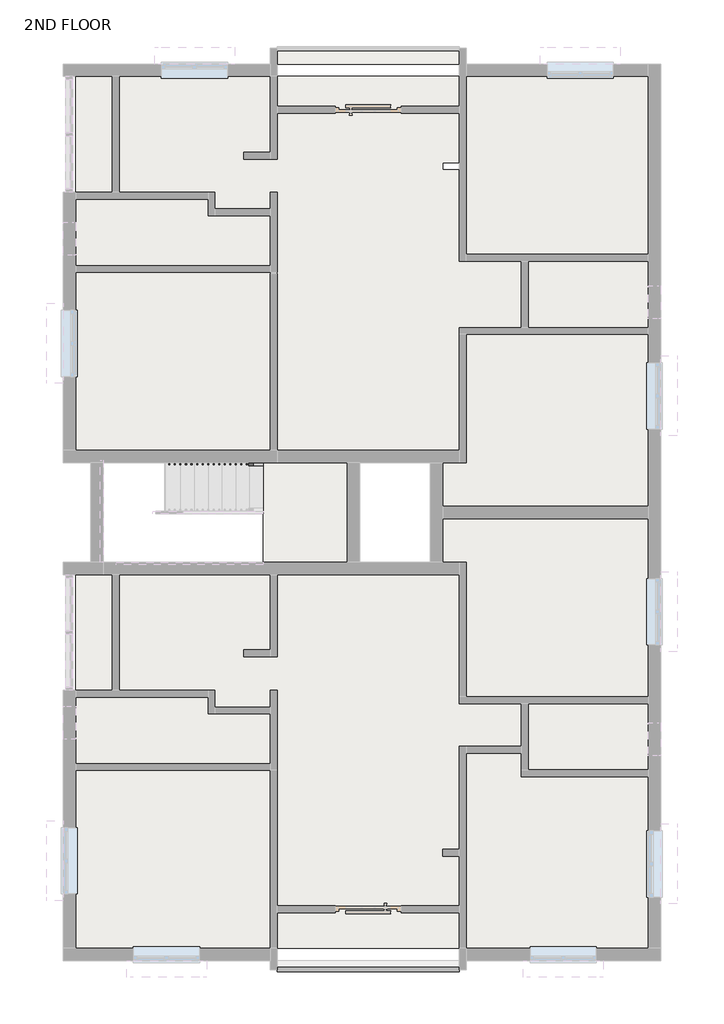
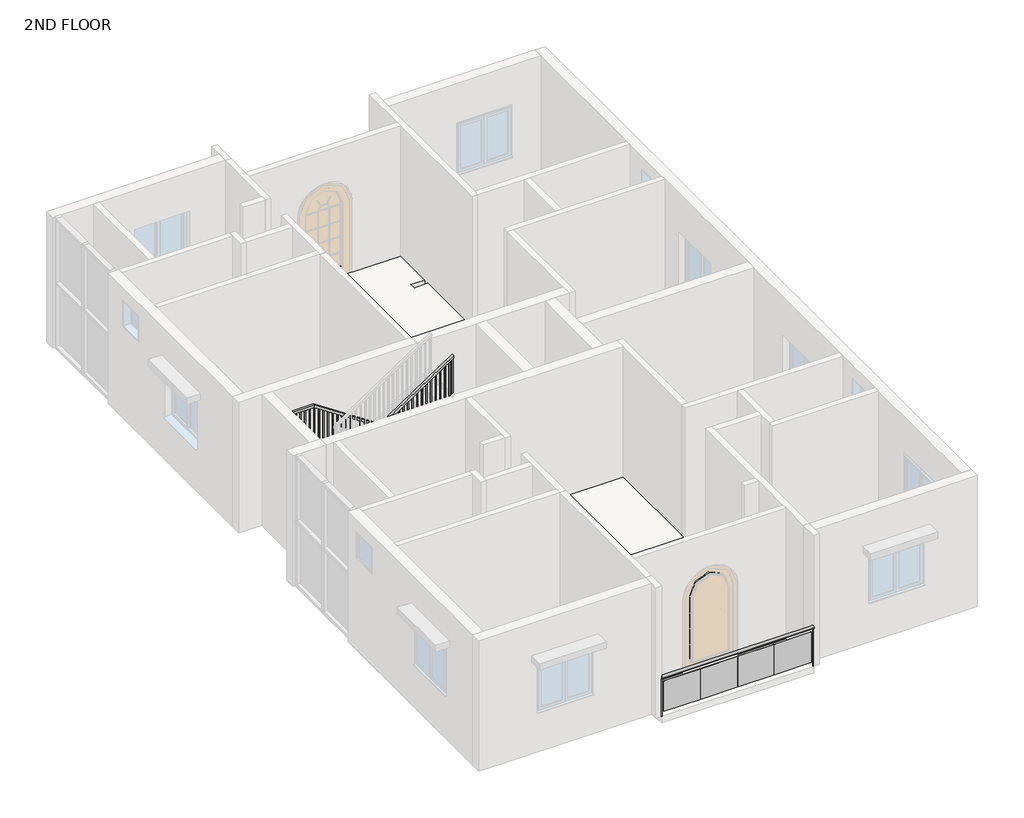
# One storey, part 3 of 4: 5 slabs, 2 railings.
"""IFC4 building model written with IfcOpenShell, lengths in millimetres."""

from ifc_helpers import new_model, si_unit, point, frame, origin, place, context, project, spatial, polyline, ellipse_curve, trimmed, outline, extrude, faceted_brep, element, save
from ifc_brep_helpers import plane_surface, extruded_surface, advanced_brep

model = new_model("IFC4")

# Units and contexts
model_context = context("Model", 3, world=origin())
ifc_project = project(units=[si_unit("LENGTHUNIT", "METRE", prefix="MILLI")], contexts=[model_context])

# Site, building, storey
site = spatial("IfcSite", under=ifc_project)
building = spatial("IfcBuilding", under=site)
storey = spatial("IfcBuildingStorey", under=building, Name="2ND FLOOR", Elevation=9144.0)

# Railings
placement = place(None, origin())
element("IfcRailing", 1, ObjectType="Glass Panel - Bottom Fill 2", at=placement, inside=storey, context=model_context, shape_type="SolidModel", body=[
    advanced_brep(
    [(-2494.0012202, -3358.1292559, 10058.4), (-2494.0012202, -3434.3292559, 10058.4), (858.7987798, -3358.1292559, 10058.4), (858.7987798, -3434.3292559, 10058.4)],
    [
        (0, 1, ellipse_curve(frame((-2494.0012202, -3396.2292559, 10058.4), z_axis=(-1.0, 0.0, 0.0), x_axis=(0.0, -1.0, 0.0)), 38.1, 28.575)),
        (1, 0, ellipse_curve(frame((-2494.0012202, -3396.2292559, 10058.4), z_axis=(-1.0, 0.0, 0.0), x_axis=(0.0, -1.0, 0.0)), 38.1, 28.575)),
        (2, 3, ellipse_curve(frame((858.7987798, -3396.2292559, 10058.4), z_axis=(1.0, 0.0, 0.0), x_axis=(0.0, -1.0, 0.0)), 38.1, 28.575)),
        (3, 2, ellipse_curve(frame((858.7987798, -3396.2292559, 10058.4), z_axis=(1.0, 0.0, 0.0), x_axis=(0.0, -1.0, 0.0)), 38.1, 28.575)),
        (0, 2),
        (3, 1),
    ],
    [
        plane_surface(frame((-2494.0012202, -3396.2292559, 10058.4), z_axis=(-1.0, 0.0, 0.0), x_axis=(0.0, 1.0, 0.0))),
        plane_surface(frame((858.7987798, -3396.2292559, 10058.4), z_axis=(1.0, 0.0, 0.0), x_axis=(0.0, 1.0, 0.0))),
        extruded_surface(trimmed(ellipse_curve(frame((858.7987798, -3396.2292559, 10058.4), z_axis=(-1.0, 0.0, 0.0), x_axis=(0.0, -1.0, 0.0)), 38.1, 28.575), [point((858.7987798, -3358.1292559, 10058.4))], [point((858.7987798, -3434.3292559, 10058.4))], True, "CARTESIAN"), (-3352.7999999999997, 0.0, 0.0), 3352.7999999999997),
        extruded_surface(trimmed(ellipse_curve(frame((858.7987798, -3396.2292559, 10058.4), z_axis=(-1.0, 0.0, 0.0), x_axis=(0.0, -1.0, 0.0)), 38.1, 28.575), [point((858.7987798, -3434.3292559, 10058.4))], [point((858.7987798, -3358.1292559, 10058.4))], True, "CARTESIAN"), (-3352.7999999999997, 0.0, 0.0), 3352.7999999999997),
    ],
    [
        (0, [[1, 2]]),
        (1, [[3, 4]]),
        (2, [[-1, 5, -4, 6]]),
        (3, [[-2, -6, -3, -5]]),
    ],
),
    extrude(outline(polyline([(-4.8012202, -3402.7644129), (-4.8012202, -3396.4144129), (807.9987798, -3396.4144129), (807.9987798, -3402.7644129), (-4.8012202, -3402.7644129)])), frame((0.0, 0.0, 9245.6), z_axis=(0.0, 0.0, 1.0), x_axis=(1.0, 0.0, 0.0)), (0.0, 0.0, 1.0), 711.2),
    extrude(outline(polyline([(-817.6012202, -3402.7644129), (-817.6012202, -3396.4144129), (-4.8012202, -3396.4144129), (-4.8012202, -3402.7644129), (-817.6012202, -3402.7644129)])), frame((0.0, 0.0, 9245.6), z_axis=(0.0, 0.0, 1.0), x_axis=(1.0, 0.0, 0.0)), (0.0, 0.0, 1.0), 711.2),
    extrude(outline(polyline([(-1630.4012202, -3402.7644129), (-1630.4012202, -3396.4144129), (-817.6012202, -3396.4144129), (-817.6012202, -3402.7644129), (-1630.4012202, -3402.7644129)])), frame((0.0, 0.0, 9245.6), z_axis=(0.0, 0.0, 1.0), x_axis=(1.0, 0.0, 0.0)), (0.0, 0.0, 1.0), 711.2),
    extrude(outline(polyline([(-2443.2012202, -3402.7644129), (-2443.2012202, -3396.4144129), (-1630.4012202, -3396.4144129), (-1630.4012202, -3402.7644129), (-2443.2012202, -3402.7644129)])), frame((0.0, 0.0, 9245.6), z_axis=(0.0, 0.0, 1.0), x_axis=(1.0, 0.0, 0.0)), (0.0, 0.0, 1.0), 711.2),
    extrude(outline(polyline([(846.0987798, -3386.7042559), (865.1487798, -3386.7042559), (865.1487798, -3405.7542559), (846.0987798, -3405.7542559), (846.0987798, -3386.7042559)])), frame((0.0, 0.0, 9144.0), z_axis=(0.0, 0.0, 1.0), x_axis=(1.0, 0.0, 0.0)), (0.0, 0.0, 1.0), 885.825),
    extrude(outline(polyline([(-2500.3512202, -3386.7042559), (-2481.3012202, -3386.7042559), (-2481.3012202, -3405.7542559), (-2500.3512202, -3405.7542559), (-2500.3512202, -3386.7042559)])), frame((0.0, 0.0, 9144.0), z_axis=(0.0, 0.0, 1.0), x_axis=(1.0, 0.0, 0.0)), (0.0, 0.0, 1.0), 885.825),
])
element("IfcRailing", 2, ObjectType="Handrail - Rectangular", at=placement, inside=storey, context=model_context, shape_type="SolidModel", body=[
    faceted_brep([(-2748.0012202, 5879.8309003, 10227.7333333), (-2748.0012202, 5879.8309003, 10166.6793317), (-2748.0012202, 5930.6309003, 10166.6793317), (-2748.0012202, 5930.6309003, 10227.7333333), (-4780.0012202, 5879.8309003, 11582.4), (-4795.3822226, 5879.8309003, 11531.6), (-4795.3822226, 5930.6309003, 11531.6), (-4780.0012202, 5930.6309003, 11582.4), (-5643.6012202, 5879.8309003, 11582.4), (-5643.6012202, 5879.8309003, 11531.6), (-5694.4012202, 5930.6309003, 11531.6), (-5694.4012202, 5930.6309003, 11582.4), (-5643.6012202, 4152.6309003, 11582.4), (-5643.6012202, 4152.6309003, 11531.6), (-5694.4012202, 4101.8309003, 11531.6), (-5694.4012202, 4101.8309003, 11582.4), (-5034.0012202, 4152.6309003, 11582.4), (-5018.6202178, 4152.6309003, 11531.6), (-5018.6202178, 4101.8309003, 11531.6), (-5034.0012202, 4101.8309003, 11582.4), (-2748.0012202, 4152.6309003, 13106.4), (-2748.0012202, 4101.8309003, 13106.4), (-2748.0012202, 4101.8309003, 13045.3459984), (-2748.0012202, 4152.6309003, 13045.3459984)], [[[0, 1, 2, 3]], [[1, 0, 4, 5]], [[2, 1, 5, 6]], [[3, 2, 6, 7]], [[0, 3, 7, 4]], [[5, 4, 8, 9]], [[6, 5, 9, 10]], [[7, 6, 10, 11]], [[4, 7, 11, 8]], [[9, 8, 12, 13]], [[10, 9, 13, 14]], [[11, 10, 14, 15]], [[8, 11, 15, 12]], [[13, 12, 16, 17]], [[14, 13, 17, 18]], [[15, 14, 18, 19]], [[12, 15, 19, 16]], [[20, 21, 22, 23]], [[17, 16, 20, 23]], [[18, 17, 23, 22]], [[19, 18, 22, 21]], [[16, 19, 21, 20]]]),
    extrude(outline(polyline([(13000.8959984, -2814.6762202), (12988.1959984, -2833.7262202), (12022.6666667, -2833.7262202), (12022.6666667, -2814.6762202), (13000.8959984, -2814.6762202)])), frame((0.0, 4117.7059003, 0.0), z_axis=(0.0, 1.0, 0.0), x_axis=(0.0, 0.0, 1.0)), (0.0, 0.0, 1.0), 19.05),
    extrude(outline(polyline([(12933.1626651, -2916.2762202), (12920.4626651, -2935.3262202), (12022.6666667, -2935.3262202), (12022.6666667, -2916.2762202), (12933.1626651, -2916.2762202)])), frame((0.0, 4117.7059003, 0.0), z_axis=(0.0, 1.0, 0.0), x_axis=(0.0, 0.0, 1.0)), (0.0, 0.0, 1.0), 19.05),
    extrude(outline(polyline([(12865.4293317, -3017.8762202), (12852.7293317, -3036.9262202), (11853.3333333, -3036.9262202), (11853.3333333, -3017.8762202), (12865.4293317, -3017.8762202)])), frame((0.0, 4117.7059003, 0.0), z_axis=(0.0, 1.0, 0.0), x_axis=(0.0, 0.0, 1.0)), (0.0, 0.0, 1.0), 19.05),
    extrude(outline(polyline([(12797.6959984, -3119.4762202), (12784.9959984, -3138.5262202), (11853.3333333, -3138.5262202), (11853.3333333, -3119.4762202), (12797.6959984, -3119.4762202)])), frame((0.0, 4117.7059003, 0.0), z_axis=(0.0, 1.0, 0.0), x_axis=(0.0, 0.0, 1.0)), (0.0, 0.0, 1.0), 19.05),
    extrude(outline(polyline([(12729.9626651, -3221.0762202), (12717.2626651, -3240.1262202), (11853.3333333, -3240.1262202), (11853.3333333, -3221.0762202), (12729.9626651, -3221.0762202)])), frame((0.0, 4117.7059003, 0.0), z_axis=(0.0, 1.0, 0.0), x_axis=(0.0, 0.0, 1.0)), (0.0, 0.0, 1.0), 19.05),
    extrude(outline(polyline([(12662.2293317, -3322.6762202), (12649.5293317, -3341.7262202), (11684.0, -3341.7262202), (11684.0, -3322.6762202), (12662.2293317, -3322.6762202)])), frame((0.0, 4117.7059003, 0.0), z_axis=(0.0, 1.0, 0.0), x_axis=(0.0, 0.0, 1.0)), (0.0, 0.0, 1.0), 19.05),
    extrude(outline(polyline([(12594.4959984, -3424.2762202), (12581.7959984, -3443.3262202), (11684.0, -3443.3262202), (11684.0, -3424.2762202), (12594.4959984, -3424.2762202)])), frame((0.0, 4117.7059003, 0.0), z_axis=(0.0, 1.0, 0.0), x_axis=(0.0, 0.0, 1.0)), (0.0, 0.0, 1.0), 19.05),
    extrude(outline(polyline([(12526.7626651, -3525.8762202), (12514.0626651, -3544.9262202), (11514.6666667, -3544.9262202), (11514.6666667, -3525.8762202), (12526.7626651, -3525.8762202)])), frame((0.0, 4117.7059003, 0.0), z_axis=(0.0, 1.0, 0.0), x_axis=(0.0, 0.0, 1.0)), (0.0, 0.0, 1.0), 19.05),
    extrude(outline(polyline([(12459.0293317, -3627.4762202), (12446.3293317, -3646.5262202), (11514.6666667, -3646.5262202), (11514.6666667, -3627.4762202), (12459.0293317, -3627.4762202)])), frame((0.0, 4117.7059003, 0.0), z_axis=(0.0, 1.0, 0.0), x_axis=(0.0, 0.0, 1.0)), (0.0, 0.0, 1.0), 19.05),
    extrude(outline(polyline([(12391.2959984, -3729.0762202), (12378.5959984, -3748.1262202), (11514.6666667, -3748.1262202), (11514.6666667, -3729.0762202), (12391.2959984, -3729.0762202)])), frame((0.0, 4117.7059003, 0.0), z_axis=(0.0, 1.0, 0.0), x_axis=(0.0, 0.0, 1.0)), (0.0, 0.0, 1.0), 19.05),
    extrude(outline(polyline([(12323.5626651, -3830.6762202), (12310.8626651, -3849.7262202), (11345.3333333, -3849.7262202), (11345.3333333, -3830.6762202), (12323.5626651, -3830.6762202)])), frame((0.0, 4117.7059003, 0.0), z_axis=(0.0, 1.0, 0.0), x_axis=(0.0, 0.0, 1.0)), (0.0, 0.0, 1.0), 19.05),
    extrude(outline(polyline([(12255.8293317, -3932.2762202), (12243.1293317, -3951.3262202), (11345.3333333, -3951.3262202), (11345.3333333, -3932.2762202), (12255.8293317, -3932.2762202)])), frame((0.0, 4117.7059003, 0.0), z_axis=(0.0, 1.0, 0.0), x_axis=(0.0, 0.0, 1.0)), (0.0, 0.0, 1.0), 19.05),
    extrude(outline(polyline([(12188.0959984, -4033.8762202), (12175.3959984, -4052.9262202), (11176.0, -4052.9262202), (11176.0, -4033.8762202), (12188.0959984, -4033.8762202)])), frame((0.0, 4117.7059003, 0.0), z_axis=(0.0, 1.0, 0.0), x_axis=(0.0, 0.0, 1.0)), (0.0, 0.0, 1.0), 19.05),
    extrude(outline(polyline([(12120.3626651, -4135.4762202), (12107.6626651, -4154.5262202), (11176.0, -4154.5262202), (11176.0, -4135.4762202), (12120.3626651, -4135.4762202)])), frame((0.0, 4117.7059003, 0.0), z_axis=(0.0, 1.0, 0.0), x_axis=(0.0, 0.0, 1.0)), (0.0, 0.0, 1.0), 19.05),
    extrude(outline(polyline([(12052.6293317, -4237.0762202), (12039.9293317, -4256.1262202), (11176.0, -4256.1262202), (11176.0, -4237.0762202), (12052.6293317, -4237.0762202)])), frame((0.0, 4117.7059003, 0.0), z_axis=(0.0, 1.0, 0.0), x_axis=(0.0, 0.0, 1.0)), (0.0, 0.0, 1.0), 19.05),
    extrude(outline(polyline([(11984.8959984, -4338.6762202), (11972.1959984, -4357.7262202), (11006.6666667, -4357.7262202), (11006.6666667, -4338.6762202), (11984.8959984, -4338.6762202)])), frame((0.0, 4117.7059003, 0.0), z_axis=(0.0, 1.0, 0.0), x_axis=(0.0, 0.0, 1.0)), (0.0, 0.0, 1.0), 19.05),
    extrude(outline(polyline([(11917.1626651, -4440.2762202), (11904.4626651, -4459.3262202), (11006.6666667, -4459.3262202), (11006.6666667, -4440.2762202), (11917.1626651, -4440.2762202)])), frame((0.0, 4117.7059003, 0.0), z_axis=(0.0, 1.0, 0.0), x_axis=(0.0, 0.0, 1.0)), (0.0, 0.0, 1.0), 19.05),
    extrude(outline(polyline([(11849.4293317, -4541.8762202), (11836.7293317, -4560.9262202), (10837.3333333, -4560.9262202), (10837.3333333, -4541.8762202), (11849.4293317, -4541.8762202)])), frame((0.0, 4117.7059003, 0.0), z_axis=(0.0, 1.0, 0.0), x_axis=(0.0, 0.0, 1.0)), (0.0, 0.0, 1.0), 19.05),
    extrude(outline(polyline([(11781.6959984, -4643.4762202), (11768.9959984, -4662.5262202), (10837.3333333, -4662.5262202), (10837.3333333, -4643.4762202), (11781.6959984, -4643.4762202)])), frame((0.0, 4117.7059003, 0.0), z_axis=(0.0, 1.0, 0.0), x_axis=(0.0, 0.0, 1.0)), (0.0, 0.0, 1.0), 19.05),
    extrude(outline(polyline([(11713.9626651, -4745.0762202), (11701.2626651, -4764.1262202), (10837.3333333, -4764.1262202), (10837.3333333, -4745.0762202), (11713.9626651, -4745.0762202)])), frame((0.0, 4117.7059003, 0.0), z_axis=(0.0, 1.0, 0.0), x_axis=(0.0, 0.0, 1.0)), (0.0, 0.0, 1.0), 19.05),
    extrude(outline(polyline([(11646.2293317, -4846.6762202), (11633.5293317, -4865.7262202), (10668.0, -4865.7262202), (10668.0, -4846.6762202), (11646.2293317, -4846.6762202)])), frame((0.0, 4117.7059003, 0.0), z_axis=(0.0, 1.0, 0.0), x_axis=(0.0, 0.0, 1.0)), (0.0, 0.0, 1.0), 19.05),
    extrude(outline(polyline([(11578.4959984, -4948.2762202), (11565.7959984, -4967.3262202), (10668.0, -4967.3262202), (10668.0, -4948.2762202), (11578.4959984, -4948.2762202)])), frame((0.0, 4117.7059003, 0.0), z_axis=(0.0, 1.0, 0.0), x_axis=(0.0, 0.0, 1.0)), (0.0, 0.0, 1.0), 19.05),
    extrude(outline(polyline([(-5068.9262202, 4117.7059003), (-5068.9262202, 4136.7559003), (-5049.8762202, 4136.7559003), (-5049.8762202, 4117.7059003), (-5068.9262202, 4117.7059003)])), frame((0.0, 0.0, 10668.0), z_axis=(0.0, 0.0, 1.0), x_axis=(1.0, 0.0, 0.0)), (0.0, 0.0, 1.0), 863.6),
    extrude(outline(polyline([(-5170.5262202, 4117.7059003), (-5170.5262202, 4136.7559003), (-5151.4762202, 4136.7559003), (-5151.4762202, 4117.7059003), (-5170.5262202, 4117.7059003)])), frame((0.0, 0.0, 10668.0), z_axis=(0.0, 0.0, 1.0), x_axis=(1.0, 0.0, 0.0)), (0.0, 0.0, 1.0), 863.6),
    extrude(outline(polyline([(-5272.1262202, 4117.7059003), (-5272.1262202, 4136.7559003), (-5253.0762202, 4136.7559003), (-5253.0762202, 4117.7059003), (-5272.1262202, 4117.7059003)])), frame((0.0, 0.0, 10668.0), z_axis=(0.0, 0.0, 1.0), x_axis=(1.0, 0.0, 0.0)), (0.0, 0.0, 1.0), 863.6),
    extrude(outline(polyline([(-5373.7262202, 4117.7059003), (-5373.7262202, 4136.7559003), (-5354.6762202, 4136.7559003), (-5354.6762202, 4117.7059003), (-5373.7262202, 4117.7059003)])), frame((0.0, 0.0, 10668.0), z_axis=(0.0, 0.0, 1.0), x_axis=(1.0, 0.0, 0.0)), (0.0, 0.0, 1.0), 863.6),
    extrude(outline(polyline([(-5475.3262202, 4117.7059003), (-5475.3262202, 4136.7559003), (-5456.2762202, 4136.7559003), (-5456.2762202, 4117.7059003), (-5475.3262202, 4117.7059003)])), frame((0.0, 0.0, 10668.0), z_axis=(0.0, 0.0, 1.0), x_axis=(1.0, 0.0, 0.0)), (0.0, 0.0, 1.0), 863.6),
    extrude(outline(polyline([(-5576.9262202, 4117.7059003), (-5576.9262202, 4136.7559003), (-5557.8762202, 4136.7559003), (-5557.8762202, 4117.7059003), (-5576.9262202, 4117.7059003)])), frame((0.0, 0.0, 10668.0), z_axis=(0.0, 0.0, 1.0), x_axis=(1.0, 0.0, 0.0)), (0.0, 0.0, 1.0), 863.6),
    extrude(outline(polyline([(-5678.5262202, 4187.5559003), (-5659.4762202, 4187.5559003), (-5659.4762202, 4168.5059003), (-5678.5262202, 4168.5059003), (-5678.5262202, 4187.5559003)])), frame((0.0, 0.0, 10668.0), z_axis=(0.0, 0.0, 1.0), x_axis=(1.0, 0.0, 0.0)), (0.0, 0.0, 1.0), 863.6),
    extrude(outline(polyline([(-5678.5262202, 4289.1559003), (-5659.4762202, 4289.1559003), (-5659.4762202, 4270.1059003), (-5678.5262202, 4270.1059003), (-5678.5262202, 4289.1559003)])), frame((0.0, 0.0, 10668.0), z_axis=(0.0, 0.0, 1.0), x_axis=(1.0, 0.0, 0.0)), (0.0, 0.0, 1.0), 863.6),
    extrude(outline(polyline([(-5678.5262202, 4390.7559003), (-5659.4762202, 4390.7559003), (-5659.4762202, 4371.7059003), (-5678.5262202, 4371.7059003), (-5678.5262202, 4390.7559003)])), frame((0.0, 0.0, 10668.0), z_axis=(0.0, 0.0, 1.0), x_axis=(1.0, 0.0, 0.0)), (0.0, 0.0, 1.0), 863.6),
    extrude(outline(polyline([(-5678.5262202, 4492.3559003), (-5659.4762202, 4492.3559003), (-5659.4762202, 4473.3059003), (-5678.5262202, 4473.3059003), (-5678.5262202, 4492.3559003)])), frame((0.0, 0.0, 10668.0), z_axis=(0.0, 0.0, 1.0), x_axis=(1.0, 0.0, 0.0)), (0.0, 0.0, 1.0), 863.6),
    extrude(outline(polyline([(-5678.5262202, 4593.9559003), (-5659.4762202, 4593.9559003), (-5659.4762202, 4574.9059003), (-5678.5262202, 4574.9059003), (-5678.5262202, 4593.9559003)])), frame((0.0, 0.0, 10668.0), z_axis=(0.0, 0.0, 1.0), x_axis=(1.0, 0.0, 0.0)), (0.0, 0.0, 1.0), 863.6),
    extrude(outline(polyline([(-5678.5262202, 4695.5559003), (-5659.4762202, 4695.5559003), (-5659.4762202, 4676.5059003), (-5678.5262202, 4676.5059003), (-5678.5262202, 4695.5559003)])), frame((0.0, 0.0, 10668.0), z_axis=(0.0, 0.0, 1.0), x_axis=(1.0, 0.0, 0.0)), (0.0, 0.0, 1.0), 863.6),
    extrude(outline(polyline([(-5678.5262202, 4797.1559003), (-5659.4762202, 4797.1559003), (-5659.4762202, 4778.1059003), (-5678.5262202, 4778.1059003), (-5678.5262202, 4797.1559003)])), frame((0.0, 0.0, 10668.0), z_axis=(0.0, 0.0, 1.0), x_axis=(1.0, 0.0, 0.0)), (0.0, 0.0, 1.0), 863.6),
    extrude(outline(polyline([(-5678.5262202, 4898.7559003), (-5659.4762202, 4898.7559003), (-5659.4762202, 4879.7059003), (-5678.5262202, 4879.7059003), (-5678.5262202, 4898.7559003)])), frame((0.0, 0.0, 10668.0), z_axis=(0.0, 0.0, 1.0), x_axis=(1.0, 0.0, 0.0)), (0.0, 0.0, 1.0), 863.6),
    extrude(outline(polyline([(-5678.5262202, 5000.3559003), (-5659.4762202, 5000.3559003), (-5659.4762202, 4981.3059003), (-5678.5262202, 4981.3059003), (-5678.5262202, 5000.3559003)])), frame((0.0, 0.0, 10668.0), z_axis=(0.0, 0.0, 1.0), x_axis=(1.0, 0.0, 0.0)), (0.0, 0.0, 1.0), 863.6),
    extrude(outline(polyline([(-5678.5262202, 5101.9559003), (-5659.4762202, 5101.9559003), (-5659.4762202, 5082.9059003), (-5678.5262202, 5082.9059003), (-5678.5262202, 5101.9559003)])), frame((0.0, 0.0, 10668.0), z_axis=(0.0, 0.0, 1.0), x_axis=(1.0, 0.0, 0.0)), (0.0, 0.0, 1.0), 863.6),
    extrude(outline(polyline([(-5678.5262202, 5203.5559003), (-5659.4762202, 5203.5559003), (-5659.4762202, 5184.5059003), (-5678.5262202, 5184.5059003), (-5678.5262202, 5203.5559003)])), frame((0.0, 0.0, 10668.0), z_axis=(0.0, 0.0, 1.0), x_axis=(1.0, 0.0, 0.0)), (0.0, 0.0, 1.0), 863.6),
    extrude(outline(polyline([(-5678.5262202, 5305.1559003), (-5659.4762202, 5305.1559003), (-5659.4762202, 5286.1059003), (-5678.5262202, 5286.1059003), (-5678.5262202, 5305.1559003)])), frame((0.0, 0.0, 10668.0), z_axis=(0.0, 0.0, 1.0), x_axis=(1.0, 0.0, 0.0)), (0.0, 0.0, 1.0), 863.6),
    extrude(outline(polyline([(-5678.5262202, 5406.7559003), (-5659.4762202, 5406.7559003), (-5659.4762202, 5387.7059003), (-5678.5262202, 5387.7059003), (-5678.5262202, 5406.7559003)])), frame((0.0, 0.0, 10668.0), z_axis=(0.0, 0.0, 1.0), x_axis=(1.0, 0.0, 0.0)), (0.0, 0.0, 1.0), 863.6),
    extrude(outline(polyline([(-5678.5262202, 5508.3559003), (-5659.4762202, 5508.3559003), (-5659.4762202, 5489.3059003), (-5678.5262202, 5489.3059003), (-5678.5262202, 5508.3559003)])), frame((0.0, 0.0, 10668.0), z_axis=(0.0, 0.0, 1.0), x_axis=(1.0, 0.0, 0.0)), (0.0, 0.0, 1.0), 863.6),
    extrude(outline(polyline([(-5678.5262202, 5609.9559003), (-5659.4762202, 5609.9559003), (-5659.4762202, 5590.9059003), (-5678.5262202, 5590.9059003), (-5678.5262202, 5609.9559003)])), frame((0.0, 0.0, 10668.0), z_axis=(0.0, 0.0, 1.0), x_axis=(1.0, 0.0, 0.0)), (0.0, 0.0, 1.0), 863.6),
    extrude(outline(polyline([(-5678.5262202, 5711.5559003), (-5659.4762202, 5711.5559003), (-5659.4762202, 5692.5059003), (-5678.5262202, 5692.5059003), (-5678.5262202, 5711.5559003)])), frame((0.0, 0.0, 10668.0), z_axis=(0.0, 0.0, 1.0), x_axis=(1.0, 0.0, 0.0)), (0.0, 0.0, 1.0), 863.6),
    extrude(outline(polyline([(-5678.5262202, 5813.1559003), (-5659.4762202, 5813.1559003), (-5659.4762202, 5794.1059003), (-5678.5262202, 5794.1059003), (-5678.5262202, 5813.1559003)])), frame((0.0, 0.0, 10668.0), z_axis=(0.0, 0.0, 1.0), x_axis=(1.0, 0.0, 0.0)), (0.0, 0.0, 1.0), 863.6),
    extrude(outline(polyline([(-5583.2762202, 5914.7559003), (-5583.2762202, 5895.7059003), (-5602.3262202, 5895.7059003), (-5602.3262202, 5914.7559003), (-5583.2762202, 5914.7559003)])), frame((0.0, 0.0, 10668.0), z_axis=(0.0, 0.0, 1.0), x_axis=(1.0, 0.0, 0.0)), (0.0, 0.0, 1.0), 863.6),
    extrude(outline(polyline([(-5481.6762202, 5914.7559003), (-5481.6762202, 5895.7059003), (-5500.7262202, 5895.7059003), (-5500.7262202, 5914.7559003), (-5481.6762202, 5914.7559003)])), frame((0.0, 0.0, 10668.0), z_axis=(0.0, 0.0, 1.0), x_axis=(1.0, 0.0, 0.0)), (0.0, 0.0, 1.0), 863.6),
    extrude(outline(polyline([(-5380.0762202, 5914.7559003), (-5380.0762202, 5895.7059003), (-5399.1262202, 5895.7059003), (-5399.1262202, 5914.7559003), (-5380.0762202, 5914.7559003)])), frame((0.0, 0.0, 10668.0), z_axis=(0.0, 0.0, 1.0), x_axis=(1.0, 0.0, 0.0)), (0.0, 0.0, 1.0), 863.6),
    extrude(outline(polyline([(-5278.4762202, 5914.7559003), (-5278.4762202, 5895.7059003), (-5297.5262202, 5895.7059003), (-5297.5262202, 5914.7559003), (-5278.4762202, 5914.7559003)])), frame((0.0, 0.0, 10668.0), z_axis=(0.0, 0.0, 1.0), x_axis=(1.0, 0.0, 0.0)), (0.0, 0.0, 1.0), 863.6),
    extrude(outline(polyline([(-5176.8762202, 5914.7559003), (-5176.8762202, 5895.7059003), (-5195.9262202, 5895.7059003), (-5195.9262202, 5914.7559003), (-5176.8762202, 5914.7559003)])), frame((0.0, 0.0, 10668.0), z_axis=(0.0, 0.0, 1.0), x_axis=(1.0, 0.0, 0.0)), (0.0, 0.0, 1.0), 863.6),
    extrude(outline(polyline([(-5075.2762202, 5914.7559003), (-5075.2762202, 5895.7059003), (-5094.3262202, 5895.7059003), (-5094.3262202, 5914.7559003), (-5075.2762202, 5914.7559003)])), frame((0.0, 0.0, 10668.0), z_axis=(0.0, 0.0, 1.0), x_axis=(1.0, 0.0, 0.0)), (0.0, 0.0, 1.0), 863.6),
    extrude(outline(polyline([(-4973.6762202, 5914.7559003), (-4973.6762202, 5895.7059003), (-4992.7262202, 5895.7059003), (-4992.7262202, 5914.7559003), (-4973.6762202, 5914.7559003)])), frame((0.0, 0.0, 10668.0), z_axis=(0.0, 0.0, 1.0), x_axis=(1.0, 0.0, 0.0)), (0.0, 0.0, 1.0), 863.6),
    extrude(outline(polyline([(-4872.0762202, 5914.7559003), (-4872.0762202, 5895.7059003), (-4891.1262202, 5895.7059003), (-4891.1262202, 5914.7559003), (-4872.0762202, 5914.7559003)])), frame((0.0, 0.0, 10668.0), z_axis=(0.0, 0.0, 1.0), x_axis=(1.0, 0.0, 0.0)), (0.0, 0.0, 1.0), 863.6),
    extrude(outline(polyline([(11514.9959984, -4770.4762202), (11527.6959984, -4789.5262202), (10668.0, -4789.5262202), (10668.0, -4770.4762202), (11514.9959984, -4770.4762202)])), frame((0.0, 5895.7059003, 0.0), z_axis=(0.0, 1.0, 0.0), x_axis=(0.0, 0.0, 1.0)), (0.0, 0.0, 1.0), 19.05),
    extrude(outline(polyline([(11447.2626651, -4668.8762202), (11459.9626651, -4687.9262202), (10498.6666667, -4687.9262202), (10498.6666667, -4668.8762202), (11447.2626651, -4668.8762202)])), frame((0.0, 5895.7059003, 0.0), z_axis=(0.0, 1.0, 0.0), x_axis=(0.0, 0.0, 1.0)), (0.0, 0.0, 1.0), 19.05),
    extrude(outline(polyline([(11379.5293317, -4567.2762202), (11392.2293317, -4586.3262202), (10498.6666667, -4586.3262202), (10498.6666667, -4567.2762202), (11379.5293317, -4567.2762202)])), frame((0.0, 5895.7059003, 0.0), z_axis=(0.0, 1.0, 0.0), x_axis=(0.0, 0.0, 1.0)), (0.0, 0.0, 1.0), 19.05),
    extrude(outline(polyline([(11311.7959984, -4465.6762202), (11324.4959984, -4484.7262202), (10329.3333333, -4484.7262202), (10329.3333333, -4465.6762202), (11311.7959984, -4465.6762202)])), frame((0.0, 5895.7059003, 0.0), z_axis=(0.0, 1.0, 0.0), x_axis=(0.0, 0.0, 1.0)), (0.0, 0.0, 1.0), 19.05),
    extrude(outline(polyline([(11244.0626651, -4364.0762202), (11256.7626651, -4383.1262202), (10329.3333333, -4383.1262202), (10329.3333333, -4364.0762202), (11244.0626651, -4364.0762202)])), frame((0.0, 5895.7059003, 0.0), z_axis=(0.0, 1.0, 0.0), x_axis=(0.0, 0.0, 1.0)), (0.0, 0.0, 1.0), 19.05),
    extrude(outline(polyline([(11176.3293317, -4262.4762202), (11189.0293317, -4281.5262202), (10329.3333333, -4281.5262202), (10329.3333333, -4262.4762202), (11176.3293317, -4262.4762202)])), frame((0.0, 5895.7059003, 0.0), z_axis=(0.0, 1.0, 0.0), x_axis=(0.0, 0.0, 1.0)), (0.0, 0.0, 1.0), 19.05),
    extrude(outline(polyline([(11108.5959984, -4160.8762202), (11121.2959984, -4179.9262202), (10160.0, -4179.9262202), (10160.0, -4160.8762202), (11108.5959984, -4160.8762202)])), frame((0.0, 5895.7059003, 0.0), z_axis=(0.0, 1.0, 0.0), x_axis=(0.0, 0.0, 1.0)), (0.0, 0.0, 1.0), 19.05),
    extrude(outline(polyline([(11040.8626651, -4059.2762202), (11053.5626651, -4078.3262202), (10160.0, -4078.3262202), (10160.0, -4059.2762202), (11040.8626651, -4059.2762202)])), frame((0.0, 5895.7059003, 0.0), z_axis=(0.0, 1.0, 0.0), x_axis=(0.0, 0.0, 1.0)), (0.0, 0.0, 1.0), 19.05),
    extrude(outline(polyline([(10973.1293317, -3957.6762202), (10985.8293317, -3976.7262202), (9990.6666667, -3976.7262202), (9990.6666667, -3957.6762202), (10973.1293317, -3957.6762202)])), frame((0.0, 5895.7059003, 0.0), z_axis=(0.0, 1.0, 0.0), x_axis=(0.0, 0.0, 1.0)), (0.0, 0.0, 1.0), 19.05),
    extrude(outline(polyline([(10905.3959984, -3856.0762202), (10918.0959984, -3875.1262202), (9990.6666667, -3875.1262202), (9990.6666667, -3856.0762202), (10905.3959984, -3856.0762202)])), frame((0.0, 5895.7059003, 0.0), z_axis=(0.0, 1.0, 0.0), x_axis=(0.0, 0.0, 1.0)), (0.0, 0.0, 1.0), 19.05),
    extrude(outline(polyline([(10837.6626651, -3754.4762202), (10850.3626651, -3773.5262202), (9990.6666667, -3773.5262202), (9990.6666667, -3754.4762202), (10837.6626651, -3754.4762202)])), frame((0.0, 5895.7059003, 0.0), z_axis=(0.0, 1.0, 0.0), x_axis=(0.0, 0.0, 1.0)), (0.0, 0.0, 1.0), 19.05),
    extrude(outline(polyline([(10769.9293317, -3652.8762202), (10782.6293317, -3671.9262202), (9821.3333333, -3671.9262202), (9821.3333333, -3652.8762202), (10769.9293317, -3652.8762202)])), frame((0.0, 5895.7059003, 0.0), z_axis=(0.0, 1.0, 0.0), x_axis=(0.0, 0.0, 1.0)), (0.0, 0.0, 1.0), 19.05),
    extrude(outline(polyline([(10702.1959984, -3551.2762202), (10714.8959984, -3570.3262202), (9821.3333333, -3570.3262202), (9821.3333333, -3551.2762202), (10702.1959984, -3551.2762202)])), frame((0.0, 5895.7059003, 0.0), z_axis=(0.0, 1.0, 0.0), x_axis=(0.0, 0.0, 1.0)), (0.0, 0.0, 1.0), 19.05),
    extrude(outline(polyline([(10634.4626651, -3449.6762202), (10647.1626651, -3468.7262202), (9652.0, -3468.7262202), (9652.0, -3449.6762202), (10634.4626651, -3449.6762202)])), frame((0.0, 5895.7059003, 0.0), z_axis=(0.0, 1.0, 0.0), x_axis=(0.0, 0.0, 1.0)), (0.0, 0.0, 1.0), 19.05),
    extrude(outline(polyline([(10566.7293317, -3348.0762202), (10579.4293317, -3367.1262202), (9652.0, -3367.1262202), (9652.0, -3348.0762202), (10566.7293317, -3348.0762202)])), frame((0.0, 5895.7059003, 0.0), z_axis=(0.0, 1.0, 0.0), x_axis=(0.0, 0.0, 1.0)), (0.0, 0.0, 1.0), 19.05),
    extrude(outline(polyline([(10498.9959984, -3246.4762202), (10511.6959984, -3265.5262202), (9652.0, -3265.5262202), (9652.0, -3246.4762202), (10498.9959984, -3246.4762202)])), frame((0.0, 5895.7059003, 0.0), z_axis=(0.0, 1.0, 0.0), x_axis=(0.0, 0.0, 1.0)), (0.0, 0.0, 1.0), 19.05),
    extrude(outline(polyline([(10431.2626651, -3144.8762202), (10443.9626651, -3163.9262202), (9482.6666667, -3163.9262202), (9482.6666667, -3144.8762202), (10431.2626651, -3144.8762202)])), frame((0.0, 5895.7059003, 0.0), z_axis=(0.0, 1.0, 0.0), x_axis=(0.0, 0.0, 1.0)), (0.0, 0.0, 1.0), 19.05),
    extrude(outline(polyline([(10363.5293317, -3043.2762202), (10376.2293317, -3062.3262202), (9482.6666667, -3062.3262202), (9482.6666667, -3043.2762202), (10363.5293317, -3043.2762202)])), frame((0.0, 5895.7059003, 0.0), z_axis=(0.0, 1.0, 0.0), x_axis=(0.0, 0.0, 1.0)), (0.0, 0.0, 1.0), 19.05),
    extrude(outline(polyline([(10295.7959984, -2941.6762202), (10308.4959984, -2960.7262202), (9313.3333333, -2960.7262202), (9313.3333333, -2941.6762202), (10295.7959984, -2941.6762202)])), frame((0.0, 5895.7059003, 0.0), z_axis=(0.0, 1.0, 0.0), x_axis=(0.0, 0.0, 1.0)), (0.0, 0.0, 1.0), 19.05),
    extrude(outline(polyline([(10228.0626651, -2840.0762202), (10240.7626651, -2859.1262202), (9313.3333333, -2859.1262202), (9313.3333333, -2840.0762202), (10228.0626651, -2840.0762202)])), frame((0.0, 5895.7059003, 0.0), z_axis=(0.0, 1.0, 0.0), x_axis=(0.0, 0.0, 1.0)), (0.0, 0.0, 1.0), 19.05),
    extrude(outline(polyline([(-5678.5262202, 4136.7559003), (-5659.4762202, 4136.7559003), (-5659.4762202, 4117.7059003), (-5678.5262202, 4117.7059003), (-5678.5262202, 4136.7559003)])), frame((0.0, 0.0, 10668.0), z_axis=(0.0, 0.0, 1.0), x_axis=(1.0, 0.0, 0.0)), (0.0, 0.0, 1.0), 863.6),
    extrude(outline(polyline([(-5659.4762202, 5914.7559003), (-5659.4762202, 5895.7059003), (-5678.5262202, 5895.7059003), (-5678.5262202, 5914.7559003), (-5659.4762202, 5914.7559003)])), frame((0.0, 0.0, 10668.0), z_axis=(0.0, 0.0, 1.0), x_axis=(1.0, 0.0, 0.0)), (0.0, 0.0, 1.0), 863.6),
    extrude(outline(polyline([(13045.3459984, -2748.0012202), (13032.6459984, -2767.0512202), (12022.6666667, -2767.0512202), (12022.6666667, -2748.0012202), (13045.3459984, -2748.0012202)])), frame((0.0, 4117.7059003, 0.0), z_axis=(0.0, 1.0, 0.0), x_axis=(0.0, 0.0, 1.0)), (0.0, 0.0, 1.0), 19.05),
    extrude(outline(polyline([(10166.6793317, -2748.0012202), (10179.3793317, -2767.0512202), (9313.3333333, -2767.0512202), (9313.3333333, -2748.0012202), (10166.6793317, -2748.0012202)])), frame((0.0, 5895.7059003, 0.0), z_axis=(0.0, 1.0, 0.0), x_axis=(0.0, 0.0, 1.0)), (0.0, 0.0, 1.0), 19.05),
])

# Slabs
element("IfcSlab", 3, ObjectType="FLOORING 6\"", at=placement, inside=storey, context=model_context, shape_type="SweptSolid", body=[
    extrude(outline(polyline([(-2621.0012202, 11645.6309003), (-3103.6012202, 11645.6309003), (-3103.6012202, 11518.6309003), (-2557.5012202, 11518.6309003), (-2494.0012202, 11518.6309003), (-2494.0012202, 13042.6309003), (858.7987798, 13042.6309003), (858.7987798, 11455.1309003), (553.9987798, 11455.1309003), (553.9987798, 11328.1309003), (858.7987798, 11328.1309003), (858.7987798, 9639.0309003), (2001.7987798, 9639.0309003), (2001.7987798, 8419.8309003), (858.7987798, 8419.8309003), (858.7987798, 6159.2309003), (-2494.0012202, 6159.2309003), (-2494.0012202, 9435.8309003), (-2494.0012202, 10909.0309003), (-2621.0012202, 10909.0309003), (-2621.0012202, 10604.2309003), (-3637.0012202, 10604.2309003), (-3637.0012202, 10909.0309003), (-6202.4012202, 10909.0309003), (-6202.4012202, 13042.6309003), (-2621.0012202, 13042.6309003), (-2621.0012202, 11645.6309003)])), frame((0.0, 0.0, 8991.6), z_axis=(0.0, 0.0, 1.0), x_axis=(1.0, 0.0, 0.0)), (0.0, 0.0, 1.0), 152.4),
])
element("IfcSlab", 4, ObjectType="FLOORING 6\"", at=placement, inside=storey, context=model_context, shape_type="SweptSolid", body=[
    extrude(outline(polyline([(4338.5987798, 13042.6309003), (4338.5987798, 9766.0309003), (985.7987798, 9766.0309003), (985.7987798, 13042.6309003), (4338.5987798, 13042.6309003)])), frame((0.0, 0.0, 8991.6), z_axis=(0.0, 0.0, 1.0), x_axis=(1.0, 0.0, 0.0)), (0.0, 0.0, 1.0), 152.4),
    extrude(outline(polyline([(4338.5987798, 9639.0309003), (4338.5987798, 8419.8309003), (2128.7987798, 8419.8309003), (2128.7987798, 9639.0309003), (4338.5987798, 9639.0309003)])), frame((0.0, 0.0, 8991.6), z_axis=(0.0, 0.0, 1.0), x_axis=(1.0, 0.0, 0.0)), (0.0, 0.0, 1.0), 152.4),
    extrude(outline(polyline([(-2621.0012202, 9435.8309003), (-2621.0012202, 6159.2309003), (-6202.4012202, 6159.2309003), (-6202.4012202, 9435.8309003), (-2621.0012202, 9435.8309003)])), frame((0.0, 0.0, 8991.6), z_axis=(0.0, 0.0, 1.0), x_axis=(1.0, 0.0, 0.0)), (0.0, 0.0, 1.0), 152.4),
    extrude(outline(polyline([(-2621.0012202, 9562.8309003), (-6202.4012202, 9562.8309003), (-6202.4012202, 10782.0309003), (-3764.0012202, 10782.0309003), (-3764.0012202, 10477.2309003), (-2621.0012202, 10477.2309003), (-2621.0012202, 9562.8309003)])), frame((0.0, 0.0, 8991.6), z_axis=(0.0, 0.0, 1.0), x_axis=(1.0, 0.0, 0.0)), (0.0, 0.0, 1.0), 152.4),
    extrude(outline(polyline([(553.9987798, 5930.6309003), (985.7987798, 5930.6309003), (985.7987798, 8292.8309003), (4338.5987798, 8292.8309003), (4338.5987798, 5130.5309003), (553.9987798, 5130.5309003), (553.9987798, 5930.6309003)])), frame((0.0, 0.0, 8991.6), z_axis=(0.0, 0.0, 1.0), x_axis=(1.0, 0.0, 0.0)), (0.0, 0.0, 1.0), 152.4),
])
element("IfcSlab", 5, ObjectType="FLOORING 6\"", at=placement, inside=storey, context=model_context, shape_type="SweptSolid", body=[
    extrude(outline(polyline([(985.7987798, 583.9309003), (2001.7987798, 583.9309003), (2001.7987798, 152.1309003), (4338.5987798, 152.1309003), (4338.5987798, -3010.1690997), (985.7987798, -3010.1690997), (985.7987798, 583.9309003)])), frame((0.0, 0.0, 8991.6), z_axis=(0.0, 0.0, 1.0), x_axis=(1.0, 0.0, 0.0)), (0.0, 0.0, 1.0), 152.4),
    extrude(outline(polyline([(-6203.9887202, -3010.1690997), (-6203.9887202, 266.4309003), (-2621.0012202, 266.4309003), (-2621.0012202, -3010.1690997), (-6203.9887202, -3010.1690997)])), frame((0.0, 0.0, 8991.6), z_axis=(0.0, 0.0, 1.0), x_axis=(1.0, 0.0, 0.0)), (0.0, 0.0, 1.0), 152.4),
    extrude(outline(polyline([(-2621.0012202, 393.4309003), (-6203.9887202, 393.4309003), (-6203.9887202, 1612.6309003), (-3764.0012202, 1612.6309003), (-3764.0012202, 1307.8309003), (-2621.0012202, 1307.8309003), (-2621.0012202, 393.4309003)])), frame((0.0, 0.0, 8991.6), z_axis=(0.0, 0.0, 1.0), x_axis=(1.0, 0.0, 0.0)), (0.0, 0.0, 1.0), 152.4),
    extrude(outline(polyline([(858.7987798, -3010.1690997), (-2494.0012202, -3010.1690997), (-2494.0012202, 1739.6309003), (-2621.0012202, 1739.6309003), (-2621.0012202, 1434.8309003), (-3637.0012202, 1434.8309003), (-3637.0012202, 1739.6309003), (-6203.9887202, 1739.6309003), (-6203.9887202, 3873.2309003), (-2621.0012202, 3873.2309003), (-2621.0012202, 2488.9309003), (-3103.6012202, 2488.9309003), (-3103.6012202, 2361.9309003), (-2494.0012202, 2361.9309003), (-2494.0012202, 3873.2309003), (858.7987798, 3873.2309003), (858.7987798, 1498.3309003), (2001.7987798, 1498.3309003), (2001.7987798, 710.9309003), (858.7987798, 710.9309003), (858.7987798, -3010.1690997)])), frame((0.0, 0.0, 8991.6), z_axis=(0.0, 0.0, 1.0), x_axis=(1.0, 0.0, 0.0)), (0.0, 0.0, 1.0), 152.4),
    extrude(outline(polyline([(985.7987798, 1625.3309003), (985.7987798, 4101.8309003), (553.9987798, 4101.8309003), (553.9987798, 4901.9309003), (4338.5987798, 4901.9309003), (4338.5987798, 1625.3309003), (985.7987798, 1625.3309003)])), frame((0.0, 0.0, 8991.6), z_axis=(0.0, 0.0, 1.0), x_axis=(1.0, 0.0, 0.0)), (0.0, 0.0, 1.0), 152.4),
    extrude(outline(polyline([(-2748.0012202, 4000.2309003), (-2748.0012202, 5981.4309003), (-2748.0012202, 6032.2309003), (-2494.0012202, 6032.2309003), (-2494.0012202, 5930.6309003), (-1198.6012202, 5930.6309003), (-1198.6012202, 4101.8309003), (-2494.0012202, 4101.8309003), (-2494.0012202, 4000.2309003), (-2748.0012202, 4000.2309003)])), frame((0.0, 0.0, 8991.6), z_axis=(0.0, 0.0, 1.0), x_axis=(1.0, 0.0, 0.0)), (0.0, 0.0, 1.0), 152.4),
])
element("IfcSlab", 6, ObjectType="bathroom tiles", at=placement, inside=storey, context=model_context, shape_type="SweptSolid", body=[
    extrude(outline(polyline([(858.7987798, 13563.3309003), (858.7987798, 13271.2309003), (-2494.0012202, 13271.2309003), (-2494.0012202, 13563.3309003), (858.7987798, 13563.3309003)])), frame((0.0, 0.0, 8991.6), z_axis=(0.0, 0.0, 1.0), x_axis=(1.0, 0.0, 0.0)), (0.0, 0.0, 1.0), 152.4),
])
element("IfcSlab", 7, ObjectType="bathroom tiles", at=placement, inside=storey, context=model_context, shape_type="SweptSolid", body=[
    extrude(outline(polyline([(4338.5987798, 1498.3309003), (4338.5987798, 279.1309003), (2128.7987798, 279.1309003), (2128.7987798, 1498.3309003), (4338.5987798, 1498.3309003)])), frame((0.0, 0.0, 8991.6), z_axis=(0.0, 0.0, 1.0), x_axis=(1.0, 0.0, 0.0)), (0.0, 0.0, 1.0), 152.4),
])

save(model, "model.ifc")

# Revit data of these elements
# Type "Glass Panel - Bottom Fill 2"
#   Assembly Code = "C2010400"
#   built-in parameter 1008612 = 0.0416667 (stored number, unit not read)
#   built-in parameter 1008611 = 0.0416667 (stored number, unit not read)
#   built-in parameter 1008609 = 0.333333 (stored number, unit not read)
#   built-in parameter 1008604 = 0.166667 (stored number, unit not read)
#   built-in parameter 1008603 = 0.166667 (stored number, unit not read)
#   Railing Height = 3' - 0"
#   built-in parameter 1008630 = 2
#   built-in parameter 1008610 = 2
#   built-in parameter 1008618 = Baluster - Square : 3/4"
# Type "Handrail - Rectangular"
#   Assembly Code = "C2010400"
#   built-in parameter 1008612 = 0.0416667 (stored number, unit not read)
#   built-in parameter 1008611 = 0.0416667 (stored number, unit not read)
#   built-in parameter 1008609 = 0.333333 (stored number, unit not read)
#   built-in parameter 1008604 = 0.166667 (stored number, unit not read)
#   built-in parameter 1008603 = 0.166667 (stored number, unit not read)
#   Railing Height = 3' - 0"
#   built-in parameter 1008630 = 2
#   built-in parameter 1008610 = 2
#   built-in parameter 1008618 = Baluster - Square : 3/4"
# Type "FLOORING 6\""
#   Assembly Code = "B1010"
#   Function = 0
#   Layers, outside or top first: 0' - 6" "MARBLE FLOORING" (function 1)
# Type "bathroom tiles"
#   Assembly Code = "B1010"
#   Function = 0
#   Layers, outside or top first: 0' - 6" "tile flooring" (function 1)
# Element 1 (IfcRailing, "Glass Panel - Bottom Fill 2")
#   Phase Created = New Construction
#   Materials on its faces: "Glass"
# Element 2 (IfcRailing, "Handrail - Rectangular")
#   Phase Created = New Construction
# Element 3 (IfcSlab, "FLOORING 6\"")
#   built-in parameter 1001955 = -1.5708 (stored number, unit not read)
#   Height Offset From Level = 0' - 0"
#   Phase Created = New Construction
#   Materials on its faces: "MARBLE FLOORING"
# Element 4 (IfcSlab, "FLOORING 6\"")
#   Height Offset From Level = 0' - 0"
#   Phase Created = New Construction
#   Materials on its faces: "MARBLE FLOORING"
# Element 5 (IfcSlab, "FLOORING 6\"")
#   built-in parameter 1001955 = 1.5708 (stored number, unit not read)
#   Height Offset From Level = 0' - 0"
#   Phase Created = New Construction
#   Materials on its faces: "MARBLE FLOORING"
# Elements 6, 7 (IfcSlab, "bathroom tiles")
#   Height Offset From Level = 0' - 0"
#   Phase Created = New Construction
#   Materials on its faces: "tile flooring"
# Materials
#   "MARBLE FLOORING": class "Generic", colour RGB 120 120 120, transparency 0, Cost = 0
#   "tile flooring": class "Generic", colour RGB 120 120 120, transparency 0, Cost = 0
#   "Glass": class "Glass", colour RGB 0 128 192, transparency 0.75, Description = "Soda Lime Glass", Cost = 0
